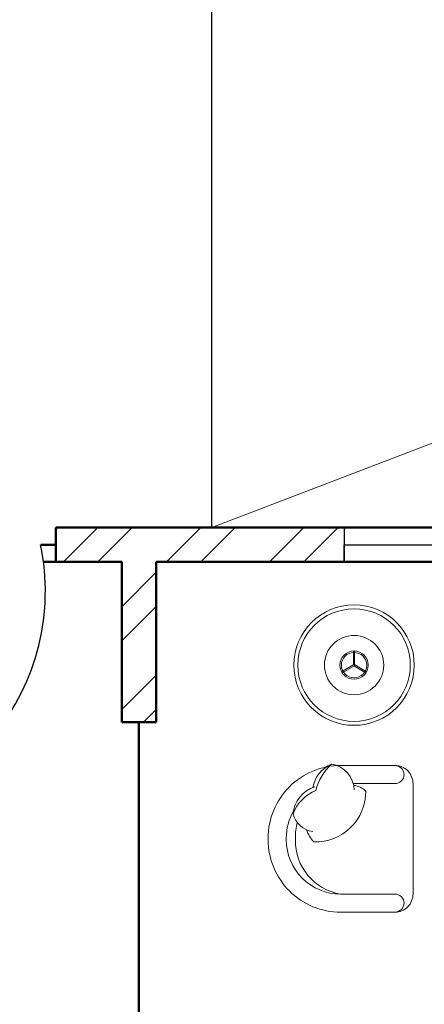
# Model space of a CAD drawing. Units: inches. Extents: x 1901 to 2863, y 888 to 2433.
# Tile 37 of 91: x 2477 to 2530, y 1603 to 1732. Entities that reach past the tile are written whole.
import ezdxf

# ---------------------------------------------------------------- set-up
doc = ezdxf.new("R2010")
doc.units = ezdxf.units.IN
for name, color, linetype, lineweight in [('A-ANNO-SYMB', 8, 'Continuous', 13), ('A-DOOR', 4, 'Continuous', 25), ('A-FLOR-HRAL', 41, 'Continuous', 25), ('A-FURN', 8, 'Continuous', 18), ('A-GLAZ', 3, 'Continuous', 25), ('A-WALL', 7, 'Continuous', 50), ('A-WALL-PATT', 8, 'Continuous', 13)]:
    doc.layers.add(name, color=color, linetype=linetype, lineweight=lineweight)

# ---------------------------------------------------------------- blocks, each defined once
blk = doc.blocks.new('WIN-60')
for p, q in [((0, 4.5), (0, 0)), ((60, 2.25), (60, 4.5)), ((60, 4.5), (60, 0)), ((0, 0), (0, 2.25)), ((0, 2.25), (60, 2.25))]:
    blk.add_line(p, q)

msp = doc.modelspace()

# ---------------------------------------------------------------- hatches: boundary and pattern name
at = {"layer": 'A-WALL-PATT'}
h = msp.add_hatch(dxfattribs=at)
h.set_pattern_fill('ANSI32', color=256)
h.paths.add_polyline_path([(2192.5, 2274.13), (2141.26, 2274.13), (2141.26, 2269.63), (2192.5, 2269.63)])
h.paths.add_polyline_path([(2259.93, 2274.13), (2216.5, 2274.13), (2216.5, 2269.63), (2255.43, 2269.63), (2255.43, 2214.63), (2250.81, 2214.63), (2250.81, 2210.13), (2259.93, 2210.13), (2259.93, 2215.13), (2271.76, 2215.13), (2271.76, 2217.38), (2271.76, 2219.63), (2259.93, 2219.63)])
h.paths.add_polyline_path([(2171.43, 2269.63), (2166.93, 2269.63), (2166.93, 2219.63), (2121.24, 2219.63), (2121.24, 2215.13), (2166.93, 2215.13), (2166.93, 2083.13), (2161.81, 2083.13), (2161.81, 2078.63), (2171.43, 2078.63), (2177, 2078.63), (2177, 2080.88), (2177, 2083.13), (2171.43, 2083.13), (2171.43, 2210.13), (2230.91, 2210.13), (2230.91, 2212.38), (2230.91, 2214.63), (2171.43, 2214.63)])
h.paths.add_polyline_path([(2117.26, 2274.13), (2089.43, 2274.13), (2089.43, 2219.63), (2081.14, 2219.63), (2081.14, 2215.13), (2089.43, 2215.13), (2098, 2215.13), (2098, 2217.38), (2098, 2219.63), (2093.93, 2219.63), (2093.93, 2269.63), (2117.26, 2269.63), (2117.26, 2271.88)])
h.paths.add_polyline_path([(2343.43, 2219.63), (2329.29, 2219.63), (2329.29, 2215.13), (2338.93, 2215.13), (2338.93, 2184.74), (2343.43, 2184.74)])
h.paths.add_polyline_path([(2338.93, 2083.13), (2329.29, 2083.13), (2208.97, 2083.13), (2208.97, 2078.63), (2338.93, 2078.63)])
h.paths.add_polyline_path([(2343.43, 2136.74), (2338.93, 2136.74), (2338.93, 1872.63), (2343.43, 1872.63)])
h.paths.add_polyline_path([(2343.43, 1863.63), (2397.68, 1863.63), (2397.68, 1821.63), (2384.14, 1821.63), (2384.14, 1812.63), (2418.33, 1812.63), (2418.33, 1817.13), (2418.33, 1821.63), (2406.68, 1821.63), (2406.68, 1863.63), (2459.5, 1863.63), (2459.5, 1821.63), (2447.14, 1821.63), (2447.14, 1812.63), (2459.5, 1812.63), (2468.5, 1812.63), (2468.5, 1872.63), (2394.43, 1872.63), (2334.43, 1872.63), (2334.43, 1812.63), (2343.43, 1812.63), (2353.25, 1812.63), (2353.25, 1821.63), (2343.43, 1821.63)])
h.paths.add_polyline_path([(2510.01, 1872.63), (2468.5, 1872.63), (2468.5, 1868.13), (2510.01, 1868.13)])
h.paths.add_polyline_path([(2514.01, 1817.13), (2468.5, 1817.13), (2468.5, 1812.63), (2482.11, 1812.63), (2482.11, 1800.61), (2486.61, 1800.61), (2486.61, 1812.63), (2514.01, 1812.63)])
h.paths.add_polyline_path([(2299.25, 1814.88), (2299.25, 1817.13), (2295.93, 1817.13), (2295.93, 1854.17), (2293.68, 1854.17), (2291.43, 1854.17), (2291.43, 1817.13), (2266.11, 1817.13), (2266.11, 1812.63), (2299.25, 1812.63)])
h.paths.add_polyline_path([(2218.11, 1817.13), (2206.46, 1817.13), (2171.43, 1817.13), (2171.43, 1949.13), (2190.1, 1949.13), (2190.1, 1953.63), (2163.47, 1953.63), (2163.47, 1949.13), (2166.93, 1949.13), (2166.93, 1817.13), (2114.3, 1817.13), (2114.3, 1812.63), (2218.11, 1812.63)])
h.paths.add_polyline_path([(2029.43, 1970.92), (2024.93, 1970.92), (2024.93, 1912.72), (2029.43, 1912.72)])
h.paths.add_polyline_path([(2132.3, 1953.63), (2113.93, 1953.63), (2113.93, 1975.89), (2111.68, 1975.89), (2109.43, 1975.89), (2109.43, 1953.63), (2029.43, 1953.63), (2029.43, 1949.13), (2132.3, 1949.13)])
h.paths.add_polyline_path([(2029.43, 1853.61), (2029.31, 1853.61), (2029.31, 1853.61), (2029.43, 1853.61), (2029.43, 1864.72), (2024.93, 1864.72), (2024.93, 1812.63), (2066.3, 1812.63), (2066.3, 1814.88), (2066.3, 1817.13), (2029.43, 1817.13)])
h.paths.add_polyline_path([(2122.93, 2010.09), (2120.68, 2010.09), (2118.43, 2010.09), (2118.43, 2006.13), (2029.43, 2006.13), (2029.43, 2001.63), (2109.43, 2001.63), (2109.43, 1998.04), (2113.93, 1998.04), (2113.93, 2001.63), (2122.93, 2001.63)])
h.paths.add_polyline_path([(2029.43, 2031.38), (2024.93, 2031.38), (2024.93, 1994.92), (2027.18, 1994.92), (2029.43, 1994.92)])
h.paths.add_polyline_path([(2029.43, 2136.74), (2024.93, 2136.74), (2024.93, 2067.38), (2027.18, 2067.38), (2029.43, 2067.38)])
h.paths.add_polyline_path([(2125.62, 2083.13), (2029.43, 2083.13), (2029.43, 2078.63), (2118.43, 2078.63), (2118.43, 2030.71), (2122.93, 2030.71), (2122.93, 2078.63), (2125.62, 2078.63)])
h.paths.add_polyline_path([(2029.43, 2215.13), (2040.47, 2215.13), (2040.47, 2217.38), (2040.47, 2219.63), (2024.93, 2219.63), (2024.93, 2184.74), (2029.43, 2184.74), (2029.43, 2187.78)])
h.paths.add_polyline_path([(2686.43, 2274.13), (2659.28, 2274.13), (2659.28, 2269.63), (2681.93, 2269.63), (2681.93, 2219.63), (2676.82, 2219.63), (2676.82, 2215.13), (2681.93, 2215.13), (2697.01, 2215.13), (2697.01, 2217.38), (2697.01, 2219.63), (2686.43, 2219.63)])
h.paths.add_polyline_path([(2609.93, 2269.63), (2635.28, 2269.63), (2635.28, 2274.13), (2571.43, 2274.13), (2571.43, 2269.63), (2605.43, 2269.63), (2605.43, 2214.63), (2549.1, 2214.63), (2549.1, 2210.13), (2605.43, 2210.13), (2605.43, 2083.13), (2601.01, 2083.13), (2601.01, 2080.88), (2601.01, 2078.63), (2609.93, 2078.63), (2616.16, 2078.63), (2616.16, 2080.88), (2616.16, 2083.13), (2609.93, 2083.13), (2609.93, 2215.13), (2651.46, 2215.13), (2651.46, 2217.38), (2651.46, 2219.63), (2609.93, 2219.63)])
h.paths.add_polyline_path([(2521.43, 2269.63), (2547.43, 2269.63), (2547.43, 2271.88), (2547.43, 2274.13), (2516.93, 2274.13), (2516.93, 2219.63), (2506.41, 2219.63), (2506.41, 2215.13), (2516.93, 2215.13), (2516.93, 2210.13), (2525.4, 2210.13), (2525.4, 2212.38), (2525.4, 2214.63), (2521.43, 2214.63)])
h.paths.add_polyline_path([(2456.01, 2219.63), (2439.43, 2219.63), (2439.43, 2187.89), (2443.93, 2187.89), (2443.93, 2215.13), (2456.01, 2215.13)])
h.paths.add_polyline_path([(2752.93, 2219.63), (2739.48, 2219.63), (2739.48, 2215.13), (2748.43, 2215.13), (2748.43, 2187.89), (2752.93, 2187.89)])
h.paths.add_polyline_path([(2752.93, 2139.89), (2748.43, 2139.89), (2748.43, 2083.13), (2648.42, 2083.13), (2648.42, 2078.63), (2654.93, 2078.63), (2654.93, 2039.44), (2659.43, 2039.44), (2659.43, 2078.63), (2748.43, 2078.63), (2748.43, 2063.43), (2752.93, 2063.43)])
h.paths.add_polyline_path([(2752.93, 2010.63), (2659.43, 2010.63), (2659.43, 2015.65), (2654.93, 2015.65), (2654.93, 2010.63), (2605.43, 2010.63), (2605.43, 1920.97), (2609.93, 1920.97), (2609.93, 2006.13), (2748.43, 2006.13), (2748.43, 1982.47), (2752.93, 1982.47)])
h.paths.add_polyline_path([(2752.93, 2027.43), (2748.43, 2027.43), (2748.43, 2010.63), (2752.93, 2010.63)])
h.paths.add_polyline_path([(2748.43, 1886.13), (2609.93, 1886.13), (2609.93, 1889.72), (2605.43, 1889.72), (2605.43, 1861.26), (2609.93, 1861.26), (2609.93, 1881.63), (2748.43, 1881.63)])
h.paths.add_polyline_path([(2456.86, 2228.83), (2498.4, 2228.83), (2498.4, 2247.49), (2456.86, 2247.49)], flags=9)
h.paths.add_polyline_path([(2038.6, 2237.42), (2080.17, 2237.42), (2080.17, 2256.08), (2038.6, 2256.08)], flags=9)
h.paths.add_polyline_path([(2292.01, 1062.39), (2539.93, 1062.39), (2539.93, 1099.49), (2292.01, 1099.49)], flags=9)
h.paths.add_polyline_path([(2424.91, 1832.25), (2448.51, 1832.25), (2448.51, 1846.68), (2424.91, 1846.68)], flags=25)
h.paths.add_polyline_path([(2359.08, 1832.25), (2382.68, 1832.25), (2382.68, 1846.68), (2359.08, 1846.68)], flags=25)
h.paths.add_polyline_path([(2352.9, 1684.8), (2367.54, 1684.8), (2367.54, 1697.17), (2352.9, 1697.17)], flags=9)
h.paths.add_polyline_path([(2079.29, 1755.83), (2169.02, 1755.83), (2169.02, 1774.37), (2079.29, 1774.37)], flags=9)
h.paths.add_polyline_path([(2404.09, 1373.86), (2404.09, 1463.59), (2385.54, 1463.59), (2385.54, 1373.86)], flags=9)
h.paths.add_polyline_path([(2268.09, 2236.37), (2309.64, 2236.37), (2309.64, 2255.03), (2268.09, 2255.03)], flags=9)
h.paths.add_polyline_path([(2575.96, 1700.95), (2665.7, 1700.95), (2665.7, 1719.5), (2575.96, 1719.5)], flags=9)
h.paths.add_polyline_path([(2302.96, 1878.47), (2329.52, 1878.47), (2329.52, 1888.78), (2302.96, 1888.78)], flags=9)
h.paths.add_polyline_path([(2097.42, 2240.58), (2126.57, 2240.58), (2126.57, 2259.23), (2097.42, 2259.23)], flags=9)
h.paths.add_polyline_path([(2208.72, 2246.12), (2237.88, 2246.12), (2237.88, 2264.78), (2208.72, 2264.78)], flags=9)
h.paths.add_polyline_path([(2038.15, 1925.96), (2076.99, 1925.96), (2076.99, 1944.62), (2038.15, 1944.62)], flags=9)
h.paths.add_polyline_path([(2239.14, 1926.67), (2288.46, 1926.67), (2288.46, 1945.33), (2239.14, 1945.33)], flags=9)
h.paths.add_polyline_path([(2175.43, 2007.33), (2212.36, 2007.33), (2212.36, 2025.99), (2175.43, 2025.99)], flags=9)
h.paths.add_polyline_path([(2225.03, 2091.79), (2263.87, 2091.79), (2263.87, 2110.45), (2225.03, 2110.45)], flags=9)
h.paths.add_polyline_path([(2035.4, 2098.48), (2074.24, 2098.48), (2074.24, 2117.14), (2035.4, 2117.14)], flags=9)
h.paths.add_polyline_path([(2050.1, 2029.21), (2083.26, 2029.21), (2083.26, 2047.87), (2050.1, 2047.87)], flags=9)
h.paths.add_polyline_path([(2069.68, 1956.72), (2098.83, 1956.72), (2098.83, 1975.38), (2069.68, 1975.38)], flags=25)
h.paths.add_polyline_path([(2328.62, 1753.34), (2361.66, 1753.34), (2361.66, 1771.99), (2328.62, 1771.99)], flags=9)
h.paths.add_polyline_path([(2395.16, 2060.89), (2395.16, 2140.65), (2378.68, 2140.65), (2378.68, 2060.89)], flags=9)
h.paths.add_polyline_path([(2463.73, 2059.02), (2492.89, 2059.02), (2492.89, 2077.68), (2463.73, 2077.68)], flags=9)
h.paths.add_polyline_path([(2458.03, 2181.54), (2496.87, 2181.54), (2496.87, 2200.19), (2458.03, 2200.19)], flags=9)
h.paths.add_polyline_path([(2527.58, 2243.07), (2556.73, 2243.07), (2556.73, 2261.73), (2527.58, 2261.73)], flags=9)
h.paths.add_polyline_path([(2694.46, 2232.77), (2736.03, 2232.77), (2736.03, 2251.42), (2694.46, 2251.42)], flags=9)
h.paths.add_polyline_path([(2637.82, 2249.22), (2666.98, 2249.22), (2666.98, 2267.88), (2637.82, 2267.88)], flags=9)
h.paths.add_polyline_path([(2623.69, 2183.54), (2662.53, 2183.54), (2662.53, 2202.2), (2623.69, 2202.2)], flags=9)
h.paths.add_polyline_path([(2691.97, 2021.5), (2725.12, 2021.5), (2725.12, 2040.16), (2691.97, 2040.16)], flags=9)
h.paths.add_polyline_path([(2621.04, 1975.91), (2662.34, 1975.91), (2662.34, 1994.57), (2621.04, 1994.57)], flags=25)
h.paths.add_polyline_path([(2479.03, 1927.62), (2519.84, 1927.62), (2519.84, 1946.28), (2479.03, 1946.28)], flags=9)
h.paths.add_polyline_path([(2670.94, 1849.08), (2716.01, 1849.08), (2716.01, 1867.73), (2670.94, 1867.73)], flags=9)
h.paths.add_polyline_path([(2523.61, 1782.96), (2550.17, 1782.96), (2550.17, 1793.26), (2523.61, 1793.26)], flags=9)
h.paths.add_polyline_path([(2450.84, 1207.33), (2492.39, 1207.33), (2492.39, 1225.99), (2450.84, 1225.99)], flags=9)
h.paths.add_polyline_path([(2527.75, 1203.84), (2556.91, 1203.84), (2556.91, 1222.5), (2527.75, 1222.5)], flags=9)
h.paths.add_polyline_path([(2639.11, 1207.2), (2668.27, 1207.2), (2668.27, 1225.86), (2639.11, 1225.86)], flags=9)
h.paths.add_polyline_path([(2692.59, 1218.97), (2734.17, 1218.97), (2734.17, 1237.62), (2692.59, 1237.62)], flags=9)
h.paths.add_polyline_path([(2669.27, 1366.33), (2708.11, 1366.33), (2708.11, 1384.99), (2669.27, 1384.99)], flags=9)
h.paths.add_polyline_path([(2463.31, 1358.03), (2502.15, 1358.03), (2502.15, 1376.69), (2463.31, 1376.69)], flags=9)
h.paths.add_polyline_path([(2494.72, 1449.96), (2531.65, 1449.96), (2531.65, 1468.62), (2494.72, 1468.62)], flags=9)
h.paths.add_polyline_path([(2675.57, 1422.16), (2708.72, 1422.16), (2708.72, 1440.81), (2675.57, 1440.81)], flags=9)
h.paths.add_polyline_path([(2685.63, 1493.89), (2714.79, 1493.89), (2714.79, 1512.55), (2685.63, 1512.55)], flags=9)
h.paths.add_polyline_path([(2686.8, 1529.91), (2725.65, 1529.91), (2725.65, 1548.57), (2686.8, 1548.57)], flags=9)
h.paths.add_polyline_path([(2503.65, 1537.99), (2552.97, 1537.99), (2552.97, 1556.65), (2503.65, 1556.65)], flags=9)
h.paths.add_polyline_path([(2291.71, 1643.5), (2318.28, 1643.5), (2318.28, 1653.81), (2291.71, 1653.81)], flags=9)
h.paths.add_polyline_path([(2450.63, 1610.52), (2477.19, 1610.52), (2477.19, 1620.82), (2450.63, 1620.82)], flags=9)
h.paths.add_polyline_path([(2359.99, 1551.81), (2422.25, 1551.81), (2422.25, 1562.12), (2359.99, 1562.12)], flags=9)
h.paths.add_polyline_path([(2280.11, 1249.01), (2321.65, 1249.01), (2321.65, 1267.66), (2280.11, 1267.66)], flags=9)
h.paths.add_polyline_path([(2164.06, 1274.23), (2193.22, 1274.23), (2193.22, 1292.89), (2164.06, 1292.89)], flags=9)
h.paths.add_polyline_path([(2118.21, 1277.69), (2151.25, 1277.69), (2151.25, 1296.35), (2118.21, 1296.35)], flags=9)
h.paths.add_polyline_path([(2031.95, 1268.53), (2073.52, 1268.53), (2073.52, 1287.19), (2031.95, 1287.19)], flags=9)
h.paths.add_polyline_path([(2050.2, 1409.08), (2089.04, 1409.08), (2089.04, 1427.74), (2050.2, 1427.74)], flags=9)
h.paths.add_polyline_path([(2243.74, 1421.03), (2282.58, 1421.03), (2282.58, 1439.69), (2243.74, 1439.69)], flags=9)
h.paths.add_polyline_path([(2190.75, 1509.77), (2231.56, 1509.77), (2231.56, 1528.43), (2190.75, 1528.43)], flags=9)
h.paths.add_polyline_path([(2058.39, 1475.42), (2091.55, 1475.42), (2091.55, 1494.07), (2058.39, 1494.07)], flags=9)
h.paths.add_polyline_path([(2062.45, 1553.09), (2091.6, 1553.09), (2091.6, 1571.75), (2062.45, 1571.75)], flags=9)
h.paths.add_polyline_path([(2219.52, 1590.37), (2266.15, 1590.37), (2266.15, 1609.02), (2219.52, 1609.02)], flags=9)
h.paths.add_polyline_path([(2041.07, 1584.19), (2079.91, 1584.19), (2079.91, 1602.85), (2041.07, 1602.85)], flags=9)
h = msp.add_hatch(dxfattribs=at)
h.set_pattern_fill('ANSI32', color=256)
h.paths.add_polyline_path([(2443.93, 2139.89), (2439.43, 2139.89), (2439.43, 2069.35), (2441.68, 2069.35), (2443.93, 2069.35), (2443.93, 2078.63), (2521.93, 2078.63), (2521.93, 2075.07), (2524.18, 2075.07), (2526.43, 2075.07), (2526.43, 2078.63), (2571.75, 2078.63), (2571.75, 2080.88), (2571.75, 2083.13), (2443.93, 2083.13)])
h.paths.add_polyline_path([(2526.43, 2054.63), (2524.18, 2054.63), (2521.93, 2054.63), (2521.93, 2030.63), (2443.93, 2030.63), (2443.93, 2045.35), (2439.43, 2045.35), (2439.43, 1983.87), (2443.93, 1983.87), (2443.93, 2026.13), (2521.93, 2026.13), (2526.43, 2026.13)])
h.paths.add_polyline_path([(2443.93, 1923.87), (2439.43, 1923.87), (2439.43, 1872.63), (2443.93, 1872.63)])
h.paths.add_polyline_path([(2636.23, 1766.13), (2609.93, 1766.13), (2609.93, 1779.79), (2605.43, 1779.79), (2605.43, 1766.13), (2486.61, 1766.13), (2486.61, 1770.67), (2482.11, 1770.67), (2482.11, 1766.13), (2482.11, 1761.63), (2636.23, 1761.63), (2636.23, 1763.88)])
h.paths.add_polyline_path([(2519.54, 1663.38), (2519.54, 1665.63), (2494.93, 1665.63), (2481.83, 1665.63), (2481.83, 1663.38), (2481.83, 1661.13), (2490.43, 1661.13), (2490.43, 1640.16), (2494.93, 1640.16), (2494.93, 1661.13), (2519.54, 1661.13)])
h.paths.add_polyline_path([(2443.93, 1712.13), (2443.93, 1716.63), (2414.46, 1716.63), (2414.46, 1712.13), (2439.43, 1712.13), (2439.43, 1545.51), (2443.93, 1545.51), (2443.93, 1661.13), (2448.47, 1661.13), (2448.47, 1665.63), (2443.93, 1665.63)])
h.paths.add_polyline_path([(2343.43, 1712.13), (2365.52, 1712.13), (2365.52, 1714.38), (2365.52, 1716.63), (2333.87, 1716.63), (2333.87, 1714.38), (2333.87, 1712.13), (2338.93, 1712.13), (2338.93, 1575.63), (2338.93, 1545.51), (2343.43, 1545.51), (2343.43, 1547.51), (2343.43, 1580.13)])
h.paths.add_polyline_path([(2752.93, 1665.63), (2579.54, 1665.63), (2579.54, 1661.13), (2615.93, 1661.13), (2615.93, 1529.13), (2598.93, 1529.13), (2598.93, 1524.63), (2623.13, 1524.63), (2623.13, 1526.88), (2623.13, 1529.13), (2620.43, 1529.13), (2620.43, 1661.13), (2748.43, 1661.13), (2748.43, 1633.5), (2752.93, 1633.5)])
h.paths.add_polyline_path([(2752.93, 1419.93), (2748.43, 1419.93), (2748.43, 1400.13), (2659.43, 1400.13), (2659.43, 1444.33), (2657.18, 1444.33), (2654.93, 1444.33), (2654.93, 1400.13), (2643.65, 1400.13), (2643.65, 1395.63), (2748.43, 1395.63), (2748.43, 1364.04), (2752.93, 1364.04)])
h.paths.add_polyline_path([(2752.93, 1492.88), (2748.43, 1492.88), (2748.43, 1476.63), (2667.43, 1476.63), (2667.43, 1479.71), (2665.18, 1479.71), (2662.93, 1479.71), (2662.93, 1476.63), (2654.93, 1476.63), (2654.93, 1469.54), (2659.43, 1469.54), (2659.43, 1472.13), (2748.43, 1472.13), (2748.43, 1455.93), (2752.93, 1455.93)])
h.paths.add_polyline_path([(2752.93, 1304.04), (2748.43, 1304.04), (2748.43, 1263.63), (2738.66, 1263.63), (2738.66, 1259.13), (2752.93, 1259.13)])
h.paths.add_polyline_path([(2685.93, 1259.13), (2695.49, 1259.13), (2695.49, 1261.38), (2695.49, 1263.63), (2677.84, 1263.63), (2677.84, 1261.38), (2677.84, 1259.13), (2681.43, 1259.13), (2681.43, 1203.63), (2653.28, 1203.63), (2653.28, 1199.13), (2685.93, 1199.13), (2685.93, 1203.63)])
h.paths.add_polyline_path([(2609.43, 1395.63), (2611.85, 1395.63), (2611.85, 1400.13), (2598.89, 1400.13), (2598.89, 1397.88), (2598.89, 1395.63), (2604.93, 1395.63), (2604.93, 1268.13), (2554.73, 1268.13), (2554.73, 1265.88), (2554.73, 1263.63), (2604.93, 1263.63), (2604.93, 1203.63), (2571.31, 1203.63), (2571.31, 1199.13), (2604.93, 1199.13), (2629.28, 1199.13), (2629.28, 1201.38), (2629.28, 1203.63), (2609.43, 1203.63), (2609.43, 1258.63), (2609.43, 1259.13), (2654.8, 1259.13), (2654.8, 1263.63), (2609.43, 1263.63)])
h.paths.add_polyline_path([(2443.93, 1304.04), (2439.43, 1304.04), (2439.43, 1259.13), (2443.93, 1259.13), (2456.16, 1259.13), (2456.16, 1261.38), (2456.16, 1263.63), (2443.93, 1263.63)])
h.paths.add_polyline_path([(2525.43, 1263.63), (2531.78, 1263.63), (2531.78, 1268.13), (2520.93, 1268.13), (2520.93, 1263.63), (2511.41, 1263.63), (2511.41, 1259.13), (2520.93, 1259.13), (2520.93, 1199.13), (2547.31, 1199.13), (2547.31, 1201.38), (2547.31, 1203.63), (2525.43, 1203.63)])
h.paths.add_polyline_path([(2443.93, 1434.84), (2439.43, 1434.84), (2439.43, 1364.04), (2441.68, 1364.04), (2443.93, 1364.04)])
h.paths.add_polyline_path([(2567.13, 1400.13), (2443.93, 1400.13), (2443.93, 1395.63), (2567.13, 1395.63)])
h.paths.add_polyline_path([(2443.93, 1545.51), (2439.43, 1545.51), (2439.43, 1494.84), (2443.93, 1494.84)])
h.paths.add_polyline_path([(2494.93, 1553.35), (2492.68, 1553.35), (2490.43, 1553.35), (2490.43, 1524.63), (2494.93, 1524.63), (2525.94, 1524.63), (2525.94, 1526.88), (2525.94, 1529.13), (2494.93, 1529.13)])
h.paths.add_polyline_path([(2752.93, 1573.5), (2748.43, 1573.5), (2748.43, 1529.13), (2657.76, 1529.13), (2657.76, 1524.63), (2662.93, 1524.63), (2662.93, 1498.63), (2667.43, 1498.63), (2667.43, 1524.63), (2748.43, 1524.63), (2748.43, 1516.88), (2752.93, 1516.88)])
h.paths.add_polyline_path([(2038.6, 2237.42), (2080.17, 2237.42), (2080.17, 2256.08), (2038.6, 2256.08)], flags=9)
h.paths.add_polyline_path([(2292.01, 1062.39), (2539.93, 1062.39), (2539.93, 1099.49), (2292.01, 1099.49)], flags=9)
h.paths.add_polyline_path([(2424.91, 1832.25), (2448.51, 1832.25), (2448.51, 1846.68), (2424.91, 1846.68)], flags=9)
h.paths.add_polyline_path([(2359.08, 1832.25), (2382.68, 1832.25), (2382.68, 1846.68), (2359.08, 1846.68)], flags=9)
h.paths.add_polyline_path([(2352.9, 1684.8), (2367.54, 1684.8), (2367.54, 1697.17), (2352.9, 1697.17)], flags=9)
h.paths.add_polyline_path([(2079.29, 1755.83), (2169.02, 1755.83), (2169.02, 1774.37), (2079.29, 1774.37)], flags=9)
h.paths.add_polyline_path([(2404.09, 1373.86), (2404.09, 1463.59), (2385.54, 1463.59), (2385.54, 1373.86)], flags=9)
h.paths.add_polyline_path([(2268.09, 2236.37), (2309.64, 2236.37), (2309.64, 2255.03), (2268.09, 2255.03)], flags=9)
h.paths.add_polyline_path([(2575.96, 1700.95), (2665.7, 1700.95), (2665.7, 1719.5), (2575.96, 1719.5)], flags=9)
h.paths.add_polyline_path([(2302.96, 1878.47), (2329.52, 1878.47), (2329.52, 1888.78), (2302.96, 1888.78)], flags=9)
h.paths.add_polyline_path([(2097.42, 2240.58), (2126.57, 2240.58), (2126.57, 2259.23), (2097.42, 2259.23)], flags=9)
h.paths.add_polyline_path([(2208.72, 2246.12), (2237.88, 2246.12), (2237.88, 2264.78), (2208.72, 2264.78)], flags=9)
h.paths.add_polyline_path([(2038.15, 1925.96), (2076.99, 1925.96), (2076.99, 1944.62), (2038.15, 1944.62)], flags=9)
h.paths.add_polyline_path([(2239.14, 1926.67), (2288.46, 1926.67), (2288.46, 1945.33), (2239.14, 1945.33)], flags=9)
h.paths.add_polyline_path([(2175.43, 2007.33), (2212.36, 2007.33), (2212.36, 2025.99), (2175.43, 2025.99)], flags=9)
h.paths.add_polyline_path([(2225.03, 2091.79), (2263.87, 2091.79), (2263.87, 2110.45), (2225.03, 2110.45)], flags=9)
h.paths.add_polyline_path([(2035.4, 2098.48), (2074.24, 2098.48), (2074.24, 2117.14), (2035.4, 2117.14)], flags=9)
h.paths.add_polyline_path([(2050.1, 2029.21), (2083.26, 2029.21), (2083.26, 2047.87), (2050.1, 2047.87)], flags=9)
h.paths.add_polyline_path([(2069.68, 1956.72), (2098.83, 1956.72), (2098.83, 1975.38), (2069.68, 1975.38)], flags=9)
h.paths.add_polyline_path([(2328.62, 1753.34), (2361.66, 1753.34), (2361.66, 1771.99), (2328.62, 1771.99)], flags=9)
h.paths.add_polyline_path([(2395.16, 2060.89), (2395.16, 2140.65), (2378.68, 2140.65), (2378.68, 2060.89)], flags=9)
h.paths.add_polyline_path([(2463.73, 2059.02), (2492.89, 2059.02), (2492.89, 2077.68), (2463.73, 2077.68)], flags=9)
h.paths.add_polyline_path([(2458.03, 2181.54), (2496.87, 2181.54), (2496.87, 2200.19), (2458.03, 2200.19)], flags=9)
h.paths.add_polyline_path([(2456.86, 2228.83), (2498.4, 2228.83), (2498.4, 2247.49), (2456.86, 2247.49)], flags=9)
h.paths.add_polyline_path([(2527.58, 2243.07), (2556.73, 2243.07), (2556.73, 2261.73), (2527.58, 2261.73)], flags=9)
h.paths.add_polyline_path([(2694.46, 2232.77), (2736.03, 2232.77), (2736.03, 2251.42), (2694.46, 2251.42)], flags=9)
h.paths.add_polyline_path([(2637.82, 2249.22), (2666.98, 2249.22), (2666.98, 2267.88), (2637.82, 2267.88)], flags=9)
h.paths.add_polyline_path([(2623.69, 2183.54), (2662.53, 2183.54), (2662.53, 2202.2), (2623.69, 2202.2)], flags=9)
h.paths.add_polyline_path([(2691.97, 2021.5), (2725.12, 2021.5), (2725.12, 2040.16), (2691.97, 2040.16)], flags=9)
h.paths.add_polyline_path([(2621.04, 1975.91), (2662.34, 1975.91), (2662.34, 1994.57), (2621.04, 1994.57)], flags=9)
h.paths.add_polyline_path([(2479.03, 1927.62), (2519.84, 1927.62), (2519.84, 1946.28), (2479.03, 1946.28)], flags=9)
h.paths.add_polyline_path([(2670.94, 1849.08), (2716.01, 1849.08), (2716.01, 1867.73), (2670.94, 1867.73)], flags=9)
h.paths.add_polyline_path([(2523.61, 1782.96), (2550.17, 1782.96), (2550.17, 1793.26), (2523.61, 1793.26)], flags=9)
h.paths.add_polyline_path([(2450.84, 1207.33), (2492.39, 1207.33), (2492.39, 1225.99), (2450.84, 1225.99)], flags=9)
h.paths.add_polyline_path([(2527.75, 1203.84), (2556.91, 1203.84), (2556.91, 1222.5), (2527.75, 1222.5)], flags=9)
h.paths.add_polyline_path([(2639.11, 1207.2), (2668.27, 1207.2), (2668.27, 1225.86), (2639.11, 1225.86)], flags=9)
h.paths.add_polyline_path([(2692.59, 1218.97), (2734.17, 1218.97), (2734.17, 1237.62), (2692.59, 1237.62)], flags=9)
h.paths.add_polyline_path([(2669.27, 1366.33), (2708.11, 1366.33), (2708.11, 1384.99), (2669.27, 1384.99)], flags=25)
h.paths.add_polyline_path([(2463.31, 1358.03), (2502.15, 1358.03), (2502.15, 1376.69), (2463.31, 1376.69)], flags=9)
h.paths.add_polyline_path([(2494.72, 1449.96), (2531.65, 1449.96), (2531.65, 1468.62), (2494.72, 1468.62)], flags=9)
h.paths.add_polyline_path([(2675.57, 1422.16), (2708.72, 1422.16), (2708.72, 1440.81), (2675.57, 1440.81)], flags=25)
h.paths.add_polyline_path([(2685.63, 1493.89), (2714.79, 1493.89), (2714.79, 1512.55), (2685.63, 1512.55)], flags=9)
h.paths.add_polyline_path([(2686.8, 1529.91), (2725.65, 1529.91), (2725.65, 1548.57), (2686.8, 1548.57)], flags=25)
h.paths.add_polyline_path([(2503.65, 1537.99), (2552.97, 1537.99), (2552.97, 1556.65), (2503.65, 1556.65)], flags=9)
h.paths.add_polyline_path([(2291.71, 1643.5), (2318.28, 1643.5), (2318.28, 1653.81), (2291.71, 1653.81)], flags=9)
h.paths.add_polyline_path([(2450.63, 1610.52), (2477.19, 1610.52), (2477.19, 1620.82), (2450.63, 1620.82)], flags=9)
h.paths.add_polyline_path([(2359.99, 1551.81), (2422.25, 1551.81), (2422.25, 1562.12), (2359.99, 1562.12)], flags=9)
h.paths.add_polyline_path([(2280.11, 1249.01), (2321.65, 1249.01), (2321.65, 1267.66), (2280.11, 1267.66)], flags=9)
h.paths.add_polyline_path([(2164.06, 1274.23), (2193.22, 1274.23), (2193.22, 1292.89), (2164.06, 1292.89)], flags=9)
h.paths.add_polyline_path([(2118.21, 1277.69), (2151.25, 1277.69), (2151.25, 1296.35), (2118.21, 1296.35)], flags=9)
h.paths.add_polyline_path([(2031.95, 1268.53), (2073.52, 1268.53), (2073.52, 1287.19), (2031.95, 1287.19)], flags=9)
h.paths.add_polyline_path([(2050.2, 1409.08), (2089.04, 1409.08), (2089.04, 1427.74), (2050.2, 1427.74)], flags=9)
h.paths.add_polyline_path([(2243.74, 1421.03), (2282.58, 1421.03), (2282.58, 1439.69), (2243.74, 1439.69)], flags=9)
h.paths.add_polyline_path([(2190.75, 1509.77), (2231.56, 1509.77), (2231.56, 1528.43), (2190.75, 1528.43)], flags=9)
h.paths.add_polyline_path([(2058.39, 1475.42), (2091.55, 1475.42), (2091.55, 1494.07), (2058.39, 1494.07)], flags=9)
h.paths.add_polyline_path([(2062.45, 1553.09), (2091.6, 1553.09), (2091.6, 1571.75), (2062.45, 1571.75)], flags=9)
h.paths.add_polyline_path([(2219.52, 1590.37), (2266.15, 1590.37), (2266.15, 1609.02), (2219.52, 1609.02)], flags=9)
h.paths.add_polyline_path([(2041.07, 1584.19), (2079.91, 1584.19), (2079.91, 1602.85), (2041.07, 1602.85)], flags=9)

# ---------------------------------------------------------------- linework, layer by layer
at = {"layer": 'A-ANNO-SYMB'}
msp.add_line((2752.93, 1761.63), (2502.24, 1665.63), dxfattribs=at)
at = {"layer": 'A-DOOR'}
msp.add_arc((2450.47, 1657.35), 29.97, 270, 11.6082, dxfattribs=at)
at = {"layer": 'A-FLOR-HRAL'}
msp.add_line((2502.24, 1665.63), (2502.24, 1761.63), dxfattribs=at)
at = {"layer": 'A-FURN', "ltscale": 0.03}
for p, q in [((2520.75, 1647.62), (2520.75, 1649.47)), ((2520.92, 1647.62), (2520.92, 1649.47)), ((2520.79, 1647.69), (2519.19, 1646.76)), ((2520.88, 1647.54), (2519.27, 1646.62)), ((2520.79, 1647.54), (2522.4, 1646.62)), ((2520.88, 1647.69), (2522.48, 1646.76))]:
    msp.add_line(p, q, dxfattribs=at)
msp.add_lwpolyline([(2528.56, 1624.88), (2528.56, 1617.66, -0.414214), (2526.19, 1615.29), (2519.08, 1615.29, -0.414214), (2509.6, 1624.76), (2509.6, 1624.88), (2509.6, 1625, -0.414214), (2519.08, 1634.48), (2526.19, 1634.48, -0.414214), (2528.56, 1632.11), (2528.56, 1624.88)], format="xyb", dxfattribs=at)
at = {"layer": 'A-FURN'}
for points in [[(2517.89, 1634.67, 0.14773), (2515.85, 1631.21, 0.213343), (2512.86, 1628.16, 0.178662)], [(2520.87, 1631.28, 0.356772), (2517.89, 1634.67, 0.249542), (2515.43, 1631.6, -9.61688)], [(2520.74, 1632.11), (2526.19, 1632.11, 0.414214), (2527.38, 1633.3), (2527.38, 1633.3, 0.414214), (2526.19, 1634.48)], [(2515.69, 1631.69, 0.306663), (2512.86, 1628.16, 0.30633), (2515.44, 1625.85, -0.872847)], [(2520.8, 1631.88, -0.165541), (2522.37, 1631.14, -0.425989), (2515.58, 1624.49, -0.121523), (2514.64, 1626.07, 7.115464)], [(2512.91, 1628.53, 0.130591), (2511.97, 1625), (2511.97, 1624.88)], [(2513.41, 1627.02, 0.072384), (2513.16, 1625), (2513.16, 1624.88)], [(2519.08, 1617.66, -0.414214), (2511.97, 1624.76), (2511.97, 1624.88)], [(2519.08, 1617.66, -0.372719), (2513.16, 1624.76), (2513.16, 1624.88)], [(2519.08, 1617.66), (2526.19, 1617.66, -0.414214), (2527.38, 1616.47), (2527.38, 1616.47, -0.414214), (2526.19, 1615.29)]]:
    msp.add_lwpolyline(points, format="xyb", dxfattribs=at)
at = {"layer": 'A-FURN', "ltscale": 0.03}
for radius in [7.88, 3.88, 1.85, 1.66]:
    msp.add_circle((2520.84, 1647.62), radius, dxfattribs=at)
at = {"layer": 'A-FURN'}
msp.add_circle((2520.84, 1647.62), 7.36, dxfattribs=at)
at = {"layer": 'A-WALL'}
for p, q in [((2752.93, 1665.63), (2481.83, 1665.63)), ((2481.83, 1661.13), (2481.83, 1665.63)), ((2481.83, 1665.63), (2481.83, 1663.38)), ((2615.93, 1665.63), (2494.93, 1665.63)), ((2481.83, 1663.38), (2479.83, 1663.38)), ((2480.2, 1661.13), (2490.43, 1661.13)), ((2490.43, 1640.16), (2490.43, 1661.13)), ((2494.93, 1661.13), (2494.93, 1640.16)), ((2494.93, 1661.13), (2615.93, 1661.13)), ((2490.43, 1640.16), (2494.93, 1640.16)), ((2492.68, 1553.35), (2492.68, 1640.16))]:
    msp.add_line(p, q, dxfattribs=at)

# ---------------------------------------------------------------- block references
at = {"layer": 'A-GLAZ'}
msp.add_blockref('WIN-60', (2519.54, 1661.13), dxfattribs=at)

doc.saveas('drawing.dxf')
